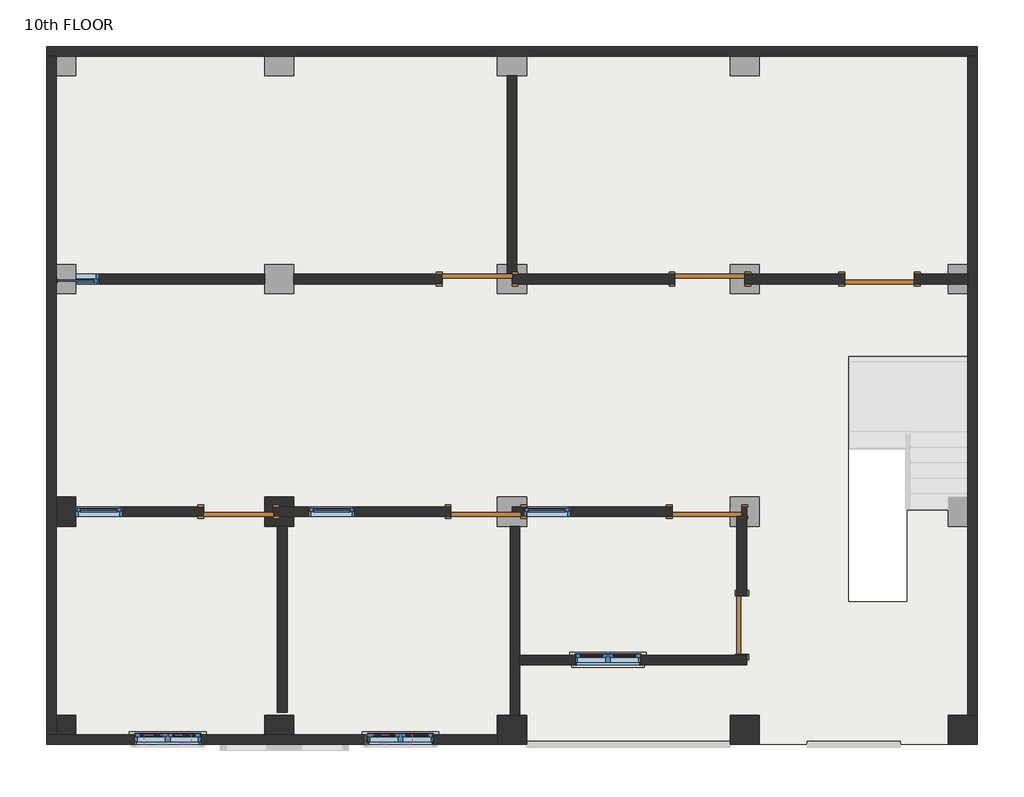
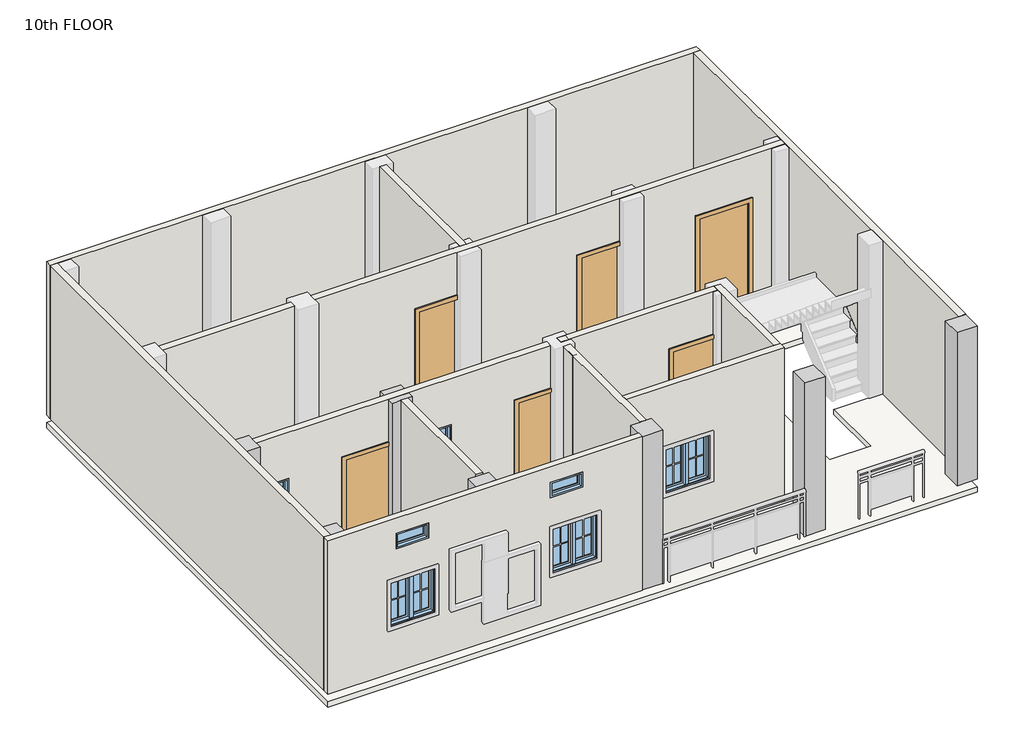
# One storey, part 1 of 2: 15 walls, 9 windows, 7 columns, 7 doors, 1 slab.
"""IFC4 building model written with IfcOpenShell, lengths in millimetres."""

from ifc_helpers import new_model, si_unit, frame, origin, place, context, project, spatial, polyline, outline, extrude, faceted_brep, transform, mapped, element, save
from components import door_e00f436c, door_a1797ceb, window_4c2727af, window_0bf3737e, window_78893e6c, window_0d9958e7

model = new_model("IFC4")

# Units and contexts
model_context = context("Model", 3, world=origin())
ifc_project = project(units=[si_unit("LENGTHUNIT", "METRE", prefix="MILLI")], contexts=[model_context])

# Site, building, storey
site = spatial("IfcSite", under=ifc_project)
building = spatial("IfcBuilding", under=site)
storey = spatial("IfcBuildingStorey", under=building, Name="10th FLOOR", Elevation=30327.6)

# Columns
placement = place(None, origin())
element("IfcColumn", 1, ObjectType="column family : column family", at=placement, inside=storey, context=model_context, shape_type="Brep", body=[
    faceted_brep([(-12576.097125, 2486.2065522, 30332.6), (-12957.097125, 2486.2065522, 30332.6), (-12957.097125, 2867.2065522, 30332.6), (-12576.097125, 2867.2065522, 30332.6), (-12576.097125, 2740.2065522, 30332.6), (-12842.797125, 2740.2065522, 30332.6), (-12842.797125, 2613.2065522, 30332.6), (-12576.097125, 2613.2065522, 30332.6), (-12576.097125, 2486.2065522, 33370.6), (-12576.097125, 2613.2065522, 33370.6), (-12957.097125, 2486.2065522, 33370.6), (-12957.097125, 2613.2065522, 33370.6), (-12957.097125, 2613.2065522, 32461.2), (-12957.097125, 2740.2065522, 32461.2), (-12957.097125, 2740.2065522, 33370.6), (-12957.097125, 2867.2065522, 33370.6), (-12576.097125, 2867.2065522, 33370.6), (-12842.797125, 2613.2065522, 32461.2), (-12842.797125, 2740.2065522, 32461.2), (-12576.097125, 2740.2065522, 33370.6)], [[[0, 1, 2, 3, 4, 5, 6, 7]], [[8, 0, 7, 9]], [[1, 0, 8, 10]], [[2, 1, 10, 11, 12, 13, 14, 15]], [[3, 2, 15, 16]], [[10, 8, 9, 11]], [[6, 17, 12, 11, 9, 7]], [[13, 18, 5, 4, 19, 14]], [[3, 16, 19, 4]], [[16, 15, 14, 19]], [[17, 18, 13, 12]], [[18, 17, 6, 5]]]),
])
element("IfcColumn", 2, ObjectType="column family : column family", at=placement, inside=storey, context=model_context, shape_type="SweptSolid", body=[
    extrude(outline(polyline([(-15433.597125, 2867.2065522), (-15433.597125, 2486.2065522), (-15687.597125, 2486.2065522), (-15687.597125, 2867.2065522), (-15433.597125, 2867.2065522)])), frame((0.0, 0.0, 30332.6), z_axis=(0.0, 0.0, 1.0), x_axis=(1.0, 0.0, 0.0)), (0.0, 0.0, 1.0), 3038.0),
])
element("IfcColumn", 3, ObjectType="column family : column family", at=placement, inside=storey, context=model_context, shape_type="SweptSolid", body=[
    extrude(outline(polyline([(-15433.597125, 9.7065522), (-15433.597125, -244.2934478), (-15687.597125, -244.2934478), (-15687.597125, 9.7065522), (-15433.597125, 9.7065522)])), frame((0.0, 0.0, 30332.6), z_axis=(0.0, 0.0, 1.0), x_axis=(1.0, 0.0, 0.0)), (0.0, 0.0, 1.0), 3038.0),
])
element("IfcColumn", 4, ObjectType="column family : column family", at=placement, inside=storey, context=model_context, shape_type="SweptSolid", body=[
    extrude(outline(polyline([(-3622.597125, 9.7065522), (-3622.597125, -371.2934478), (-4003.597125, -371.2934478), (-4003.597125, 9.7065522), (-3622.597125, 9.7065522)])), frame((0.0, 0.0, 30332.6), z_axis=(0.0, 0.0, 1.0), x_axis=(1.0, 0.0, 0.0)), (0.0, 0.0, 1.0), 3038.0),
])
element("IfcColumn", 5, ObjectType="column family : column family", at=placement, inside=storey, context=model_context, shape_type="SweptSolid", body=[
    extrude(outline(polyline([(-6480.097125, 9.7065522), (-6480.097125, -371.2934478), (-6861.097125, -371.2934478), (-6861.097125, 9.7065522), (-6480.097125, 9.7065522)])), frame((0.0, 0.0, 30332.6), z_axis=(0.0, 0.0, 1.0), x_axis=(1.0, 0.0, 0.0)), (0.0, 0.0, 1.0), 3038.0),
])
element("IfcColumn", 6, ObjectType="column family : column family", at=placement, inside=storey, context=model_context, shape_type="SweptSolid", body=[
    extrude(outline(polyline([(-9528.097125, 9.7065522), (-9528.097125, -371.2934478), (-9909.097125, -371.2934478), (-9909.097125, 9.7065522), (-9528.097125, 9.7065522)])), frame((0.0, 0.0, 30332.6), z_axis=(0.0, 0.0, 1.0), x_axis=(1.0, 0.0, 0.0)), (0.0, 0.0, 1.0), 3038.0),
])
element("IfcColumn", 7, ObjectType="column family : column family", at=placement, inside=storey, context=model_context, shape_type="SweptSolid", body=[
    extrude(outline(polyline([(-12957.097125, 9.7065522), (-12576.097125, 9.7065522), (-12576.097125, -244.2934478), (-12957.097125, -244.2934478), (-12957.097125, 9.7065522)])), frame((0.0, 0.0, 30332.6), z_axis=(0.0, 0.0, 1.0), x_axis=(1.0, 0.0, 0.0)), (0.0, 0.0, 1.0), 3038.0),
])

# Doors
door_shape = door_e00f436c(model_context)
element("IfcDoor", 8, ObjectType="Single-Flush : 30\" x 80\"", at=placement, inside=storey, context=model_context, shape_type="MappedRepresentation", body=[
    mapped(door_shape, transform((-6708.697125, 1190.8065522, 30327.6), x_axis=(0.0, -1.0, 0.0), y_axis=(1.0, 0.0, 0.0), z_axis=(0.0, 0.0, 1.0))),
])
door_2_shape = door_a1797ceb(model_context)
element("IfcDoor", 9, ObjectType="Single-Flush : 36\" x 84\"", at=placement, inside=storey, context=model_context, shape_type="MappedRepresentation", body=[
    mapped(door_2_shape, transform((-10175.797125, 5724.7065522, 30327.6), x_axis=(1.0, 0.0, 0.0), y_axis=(0.0, 1.0, 0.0), z_axis=(0.0, 0.0, 1.0))),
])
element("IfcDoor", 10, ObjectType="Single-Flush : 36\" x 84\"", at=placement, inside=storey, context=model_context, shape_type="MappedRepresentation", body=[
    mapped(door_2_shape, transform((-10061.497125, 2676.7065522, 30327.6), x_axis=(-1.0, 0.0, 0.0), y_axis=(0.0, -1.0, 0.0), z_axis=(0.0, 0.0, 1.0))),
])
element("IfcDoor", 11, ObjectType="Single-Flush : 36\" x 84\"", at=placement, inside=storey, context=model_context, shape_type="MappedRepresentation", body=[
    mapped(door_2_shape, transform((-13299.997125, 2676.7065522, 30327.6), x_axis=(-1.0, 0.0, 0.0), y_axis=(0.0, -1.0, 0.0), z_axis=(0.0, 0.0, 1.0))),
])
element("IfcDoor", 12, ObjectType="Single-Flush : 36\" x 84\"", at=placement, inside=storey, context=model_context, shape_type="MappedRepresentation", body=[
    mapped(door_2_shape, transform((-7127.797125, 5724.7065522, 30327.6), x_axis=(1.0, 0.0, 0.0), y_axis=(0.0, 1.0, 0.0), z_axis=(0.0, 0.0, 1.0))),
])
element("IfcDoor", 13, ObjectType="Single-Flush : 36\" x 84\"", at=placement, inside=storey, context=model_context, shape_type="MappedRepresentation", body=[
    mapped(door_2_shape, transform((-7165.897125, 2676.7065522, 30327.6), x_axis=(-1.0, 0.0, 0.0), y_axis=(0.0, -1.0, 0.0), z_axis=(0.0, 0.0, 1.0))),
])
element("IfcDoor", 14, ObjectType="Single-Flush : 36\" x 84\"", at=placement, inside=storey, context=model_context, shape_type="MappedRepresentation", body=[
    mapped(door_2_shape, transform((-4905.297125, 5724.7065522, 30327.6), x_axis=(-1.0, 0.0, 0.0), y_axis=(0.0, -1.0, 0.0), z_axis=(0.0, 0.0, 1.0))),
])

# Slab
element("IfcSlab", 15, ObjectType="Generic - 4\"", at=placement, inside=storey, context=model_context, shape_type="SweptSolid", body=[
    extrude(outline(polyline([(-3622.597125, 8772.7065522), (-3622.597125, -371.2934478), (-15814.597125, -371.2934478), (-15814.597125, 8772.7065522), (-3622.597125, 8772.7065522)]), holes=[polyline([(-3734.357125, 4711.0719226), (-5310.2646464, 4711.0719226), (-5310.2646464, 1502.3126957), (-4547.7736682, 1502.3126957), (-4547.7736682, 2699.911213), (-3734.357125, 2699.911213), (-3734.357125, 4711.0719226)])]), frame((0.0, 0.0, 30073.6), z_axis=(0.0, 0.0, 1.0), x_axis=(1.0, 0.0, 0.0)), (0.0, 0.0, 1.0), 101.6),
])

# Walls
element("IfcWall", 16, ObjectType="Generic - 5\"", at=placement, inside=storey, context=model_context, shape_type="Brep", body=[
    faceted_brep([(-15814.597125, 8645.7065522, 30327.6), (-15687.597125, 8645.7065522, 30327.6), (-3749.597125, 8645.7065522, 30327.6), (-3622.597125, 8645.7065522, 30327.6), (-3622.597125, 8645.7065522, 33375.6), (-3749.597125, 8645.7065522, 33375.6), (-15687.597125, 8645.7065522, 33375.6), (-15814.597125, 8645.7065522, 33375.6), (-15814.597125, 8772.7065522, 30327.6), (-15814.597125, 8772.7065522, 33375.6), (-3622.597125, 8772.7065522, 33375.6), (-3622.597125, 8772.7065522, 30327.6)], [[[0, 1, 2, 3, 4, 5, 6, 7]], [[8, 9, 10, 11]], [[3, 2, 1, 0, 8, 11]], [[7, 6, 5, 4, 10, 9]], [[4, 3, 11, 10]], [[0, 7, 9, 8]]]),
])
element("IfcWall", 17, ObjectType="Generic - 5\"", at=placement, inside=storey, context=model_context, shape_type="Brep", body=[
    faceted_brep([(-3749.597125, 8645.7065522, 30327.6), (-3749.597125, 5788.2065522, 30327.6), (-3749.597125, 5661.2065522, 30327.6), (-3749.597125, 9.7065522, 30327.6), (-3749.597125, 9.7065522, 33375.6), (-3749.597125, 5661.2065522, 33375.6), (-3749.597125, 5788.2065522, 33375.6), (-3749.597125, 8645.7065522, 33375.6), (-3622.597125, 8645.7065522, 30327.6), (-3622.597125, 8645.7065522, 33375.6), (-3622.597125, 9.7065522, 33375.6), (-3622.597125, 9.7065522, 33370.6), (-3622.597125, 9.7065522, 30332.6), (-3622.597125, 9.7065522, 30327.6)], [[[0, 1, 2, 3, 4, 5, 6, 7]], [[8, 9, 10, 11, 12, 13]], [[3, 2, 1, 0, 8, 13]], [[4, 3, 13, 12, 11, 10]], [[7, 6, 5, 4, 10, 9]], [[0, 7, 9, 8]]]),
])
element("IfcWall", 18, ObjectType="Generic - 5\"", at=placement, inside=storey, context=model_context, shape_type="Brep", body=[
    faceted_brep([(-9909.097125, -244.2934478, 30327.6), (-15687.597125, -244.2934478, 30327.6), (-15814.597125, -244.2934478, 30327.6), (-15814.597125, -244.2934478, 33375.6), (-15687.597125, -244.2934478, 33375.6), (-9909.097125, -244.2934478, 33375.6), (-13795.297125, -244.2934478, 32156.4), (-14658.897125, -244.2934478, 32156.4), (-14658.897125, -244.2934478, 31242.0), (-13795.297125, -244.2934478, 31242.0), (-10747.297125, -244.2934478, 32156.4), (-11610.897125, -244.2934478, 32156.4), (-11610.897125, -244.2934478, 31242.0), (-10747.297125, -244.2934478, 31242.0), (-13922.297125, -244.2934478, 33070.8), (-14531.897125, -244.2934478, 33070.8), (-14531.897125, -244.2934478, 32766.0), (-13922.297125, -244.2934478, 32766.0), (-11026.697125, -244.2934478, 33070.8), (-11636.297125, -244.2934478, 33070.8), (-11636.297125, -244.2934478, 32766.0), (-11026.697125, -244.2934478, 32766.0), (-9909.097125, -371.2934478, 30327.6), (-9909.097125, -371.2934478, 30332.6), (-9909.097125, -371.2934478, 33370.6), (-9909.097125, -371.2934478, 33375.6), (-15814.597125, -371.2934478, 33375.6), (-15814.597125, -371.2934478, 30327.6), (-13795.297125, -371.2934478, 32156.4), (-13795.297125, -371.2934478, 31242.0), (-14658.897125, -371.2934478, 31242.0), (-14658.897125, -371.2934478, 32156.4), (-10747.297125, -371.2934478, 32156.4), (-10747.297125, -371.2934478, 31242.0), (-11610.897125, -371.2934478, 31242.0), (-11610.897125, -371.2934478, 32156.4), (-13922.297125, -371.2934478, 33070.8), (-13922.297125, -371.2934478, 32766.0), (-14531.897125, -371.2934478, 32766.0), (-14531.897125, -371.2934478, 33070.8), (-11026.697125, -371.2934478, 33070.8), (-11026.697125, -371.2934478, 32766.0), (-11636.297125, -371.2934478, 32766.0), (-11636.297125, -371.2934478, 33070.8)], [[[0, 1, 2, 3, 4, 5], [6, 7, 8, 9], [10, 11, 12, 13], [14, 15, 16, 17], [18, 19, 20, 21]], [[22, 23, 24, 25, 26, 27], [28, 29, 30, 31], [32, 33, 34, 35], [36, 37, 38, 39], [40, 41, 42, 43]], [[2, 1, 0, 22, 27]], [[5, 4, 3, 26, 25]], [[0, 5, 25, 24, 23, 22]], [[3, 2, 27, 26]], [[29, 28, 6, 9]], [[30, 29, 9, 8]], [[31, 30, 8, 7]], [[28, 31, 7, 6]], [[33, 32, 10, 13]], [[34, 33, 13, 12]], [[35, 34, 12, 11]], [[32, 35, 11, 10]], [[37, 36, 14, 17]], [[38, 37, 17, 16]], [[39, 38, 16, 15]], [[36, 39, 15, 14]], [[41, 40, 18, 21]], [[42, 41, 21, 20]], [[43, 42, 20, 19]], [[40, 43, 19, 18]]]),
])
element("IfcWall", 19, ObjectType="Generic - 5\"", at=placement, inside=storey, context=model_context, shape_type="Brep", body=[
    faceted_brep([(-15687.597125, -244.2934478, 30327.6), (-15687.597125, 8645.7065522, 30327.6), (-15687.597125, 8645.7065522, 30332.6), (-15687.597125, 8645.7065522, 33370.6), (-15687.597125, 8645.7065522, 33375.6), (-15687.597125, -244.2934478, 33375.6), (-15687.597125, -244.2934478, 33370.6), (-15687.597125, -244.2934478, 30332.6), (-15814.597125, -244.2934478, 30327.6), (-15814.597125, -244.2934478, 33375.6), (-15814.597125, 8645.7065522, 33375.6), (-15814.597125, 8645.7065522, 30327.6)], [[[0, 1, 2, 3, 4, 5, 6, 7]], [[8, 9, 10, 11]], [[1, 0, 8, 11]], [[5, 4, 10, 9]], [[4, 3, 2, 1, 11, 10]], [[0, 7, 6, 5, 9, 8]]]),
])
element("IfcWall", 20, ObjectType="Generic - 5\"", at=placement, inside=storey, context=model_context, shape_type="SweptSolid", body=[
    extrude(outline(polyline([(30327.6, -15433.597125), (30327.6, -12957.097125), (33375.6, -12957.097125), (33375.6, -15433.597125), (32461.2, -15433.597125), (32461.2, -15128.797125), (30632.4, -15128.797125), (30632.4, -15433.597125), (30327.6, -15433.597125)])), frame((0.0, 5661.2065522, 0.0), z_axis=(0.0, 1.0, 0.0), x_axis=(0.0, 0.0, 1.0)), (0.0, 0.0, 1.0), 127.0),
])
element("IfcWall", 21, ObjectType="Generic - 5\"", at=placement, inside=storey, context=model_context, shape_type="Brep", body=[
    faceted_brep([(-9782.097125, 8391.7065522, 30327.6), (-9782.097125, 5788.2065522, 30327.6), (-9782.097125, 5788.2065522, 30332.6), (-9782.097125, 5788.2065522, 32461.2), (-9782.097125, 5788.2065522, 33370.6), (-9782.097125, 5788.2065522, 33375.6), (-9782.097125, 8391.7065522, 33375.6), (-9655.097125, 8391.7065522, 30327.6), (-9655.097125, 8391.7065522, 33375.6), (-9655.097125, 5788.2065522, 33375.6), (-9655.097125, 5788.2065522, 33370.6), (-9655.097125, 5788.2065522, 30332.6), (-9655.097125, 5788.2065522, 30327.6), (-9718.597125, 5788.2065522, 30327.6)], [[[0, 1, 2, 3, 4, 5, 6]], [[7, 8, 9, 10, 11, 12]], [[1, 0, 7, 12, 13]], [[6, 5, 9, 8]], [[0, 6, 8, 7]], [[5, 4, 3, 2, 1, 13, 12, 11, 10, 9]]]),
])
element("IfcWall", 22, ObjectType="Generic - 5\"", at=placement, inside=storey, context=model_context, shape_type="Brep", body=[
    faceted_brep([(-6670.597125, 5661.2065522, 30327.6), (-5362.497125, 5661.2065522, 30327.6), (-5362.497125, 5661.2065522, 32461.2), (-4448.097125, 5661.2065522, 32461.2), (-4448.097125, 5661.2065522, 30327.6), (-3749.597125, 5661.2065522, 30327.6), (-3749.597125, 5661.2065522, 30332.6), (-3749.597125, 5661.2065522, 33370.6), (-3749.597125, 5661.2065522, 33375.6), (-12576.097125, 5661.2065522, 33375.6), (-12576.097125, 5661.2065522, 30327.6), (-10632.997125, 5661.2065522, 30327.6), (-10632.997125, 5661.2065522, 32461.2), (-9909.097125, 5661.2065522, 32461.2), (-9718.597125, 5661.2065522, 32461.2), (-9718.597125, 5661.2065522, 30332.6), (-9718.597125, 5661.2065522, 30327.6), (-7584.997125, 5661.2065522, 30327.6), (-7584.997125, 5661.2065522, 32461.2), (-6861.097125, 5661.2065522, 32461.2), (-6670.597125, 5661.2065522, 32461.2), (-6670.597125, 5661.2065522, 30332.6), (-5362.497125, 5788.2065522, 32461.2), (-5362.497125, 5788.2065522, 30327.6), (-6670.597125, 5788.2065522, 30327.6), (-6670.597125, 5788.2065522, 30332.6), (-6670.597125, 5788.2065522, 32461.2), (-6861.097125, 5788.2065522, 32461.2), (-7584.997125, 5788.2065522, 32461.2), (-7584.997125, 5788.2065522, 30327.6), (-9655.097125, 5788.2065522, 30327.6), (-9718.597125, 5788.2065522, 30327.6), (-9718.597125, 5788.2065522, 30332.6), (-9718.597125, 5788.2065522, 32461.2), (-9782.097125, 5788.2065522, 32461.2), (-9909.097125, 5788.2065522, 32461.2), (-10632.997125, 5788.2065522, 32461.2), (-10632.997125, 5788.2065522, 30327.6), (-12576.097125, 5788.2065522, 30327.6), (-12576.097125, 5788.2065522, 33375.6), (-9782.097125, 5788.2065522, 33375.6), (-9655.097125, 5788.2065522, 33375.6), (-3749.597125, 5788.2065522, 33375.6), (-3749.597125, 5788.2065522, 33370.6), (-3749.597125, 5788.2065522, 30332.6), (-3749.597125, 5788.2065522, 30327.6), (-4448.097125, 5788.2065522, 30327.6), (-4448.097125, 5788.2065522, 32461.2)], [[[0, 1, 2, 3, 4, 5, 6, 7, 8, 9, 10, 11, 12, 13, 14, 15, 16, 17, 18, 19, 20, 21]], [[22, 23, 24, 25, 26, 27, 28, 29, 30, 31, 32, 33, 34, 35, 36, 37, 38, 39, 40, 41, 42, 43, 44, 45, 46, 47]], [[11, 10, 38, 37]], [[17, 16, 31, 30, 29]], [[46, 45, 5, 4]], [[24, 23, 1, 0]], [[9, 8, 42, 41, 40, 39]], [[10, 9, 39, 38]], [[8, 7, 6, 5, 45, 44, 43, 42]], [[33, 32, 31, 16, 15, 14]], [[36, 35, 34, 33, 14, 13, 12]], [[37, 36, 12, 11]], [[26, 25, 24, 0, 21, 20]], [[28, 27, 26, 20, 19, 18]], [[29, 28, 18, 17]], [[2, 1, 23, 22]], [[3, 2, 22, 47]], [[4, 3, 47, 46]]]),
])
element("IfcWall", 23, ObjectType="Generic - 5\"", at=placement, inside=storey, context=model_context, shape_type="Brep", body=[
    faceted_brep([(-14823.997125, 2613.2065522, 30632.4), (-15433.597125, 2613.2065522, 30632.4), (-15433.597125, 2613.2065522, 30327.6), (-13757.197125, 2613.2065522, 30327.6), (-13757.197125, 2613.2065522, 32461.2), (-12957.097125, 2613.2065522, 32461.2), (-12842.797125, 2613.2065522, 32461.2), (-12842.797125, 2613.2065522, 30332.6), (-12842.797125, 2613.2065522, 30327.6), (-10518.697125, 2613.2065522, 30327.6), (-10518.697125, 2613.2065522, 32461.2), (-9909.097125, 2613.2065522, 32461.2), (-9909.097125, 2613.2065522, 33375.6), (-15433.597125, 2613.2065522, 33375.6), (-15433.597125, 2613.2065522, 32461.2), (-14823.997125, 2613.2065522, 32461.2), (-12385.597125, 2613.2065522, 32461.2), (-11775.997125, 2613.2065522, 32461.2), (-11775.997125, 2613.2065522, 30632.4), (-12385.597125, 2613.2065522, 30632.4), (-15433.597125, 2740.2065522, 30327.6), (-15433.597125, 2740.2065522, 30632.4), (-14823.997125, 2740.2065522, 30632.4), (-14823.997125, 2740.2065522, 32461.2), (-15433.597125, 2740.2065522, 32461.2), (-15433.597125, 2740.2065522, 33375.6), (-9909.097125, 2740.2065522, 33375.6), (-9909.097125, 2740.2065522, 32461.2), (-10518.697125, 2740.2065522, 32461.2), (-10518.697125, 2740.2065522, 30327.6), (-12842.797125, 2740.2065522, 30327.6), (-12842.797125, 2740.2065522, 30332.6), (-12842.797125, 2740.2065522, 32461.2), (-12957.097125, 2740.2065522, 32461.2), (-13757.197125, 2740.2065522, 32461.2), (-13757.197125, 2740.2065522, 30327.6), (-12385.597125, 2740.2065522, 32461.2), (-12385.597125, 2740.2065522, 30632.4), (-11775.997125, 2740.2065522, 30632.4), (-11775.997125, 2740.2065522, 32461.2)], [[[0, 1, 2, 3, 4, 5, 6, 7, 8, 9, 10, 11, 12, 13, 14, 15], [16, 17, 18, 19]], [[20, 21, 22, 23, 24, 25, 26, 27, 28, 29, 30, 31, 32, 33, 34, 35], [36, 37, 38, 39]], [[30, 29, 9, 8]], [[20, 35, 3, 2]], [[26, 12, 11, 27]], [[13, 12, 26, 25]], [[14, 13, 25, 24]], [[2, 1, 21, 20]], [[28, 10, 9, 29]], [[10, 28, 27, 11]], [[4, 3, 35, 34]], [[6, 5, 4, 34, 33, 32]], [[8, 7, 6, 32, 31, 30]], [[22, 21, 1, 0]], [[23, 22, 0, 15]], [[24, 23, 15, 14]], [[37, 36, 16, 19]], [[38, 37, 19, 18]], [[39, 38, 18, 17]], [[36, 39, 17, 16]]]),
])
element("IfcWall", 24, ObjectType="Generic - 5\"", at=placement, inside=storey, context=model_context, shape_type="Brep", body=[
    faceted_brep([(-9616.997125, 9.7065522, 30327.6), (-9616.997125, 670.1065522, 30327.6), (-9616.997125, 797.1065522, 30327.6), (-9616.997125, 2486.2065522, 30327.6), (-9616.997125, 2486.2065522, 33375.6), (-9616.997125, 797.1065522, 33375.6), (-9616.997125, 670.1065522, 33375.6), (-9616.997125, 9.7065522, 33375.6), (-9743.997125, 9.7065522, 30327.6), (-9743.997125, 9.7065522, 33375.6), (-9743.997125, 2486.2065522, 33375.6), (-9743.997125, 2486.2065522, 30327.6)], [[[0, 1, 2, 3, 4, 5, 6, 7]], [[8, 9, 10, 11]], [[3, 2, 1, 0, 8, 11]], [[4, 3, 11, 10]], [[7, 6, 5, 4, 10, 9]], [[0, 7, 9, 8]]]),
])
element("IfcWall", 25, ObjectType="Generic - 5\"", at=placement, inside=storey, context=model_context, shape_type="SweptSolid", body=[
    extrude(outline(polyline([(-9743.997125, 2181.4065522), (-9743.997125, 2486.2065522), (-9616.997125, 2486.2065522), (-9616.997125, 2181.4065522), (-9743.997125, 2181.4065522)])), frame((0.0, 0.0, 30327.6), z_axis=(0.0, 0.0, 1.0), x_axis=(1.0, 0.0, 0.0)), (0.0, 0.0, 1.0), 3048.0),
])
element("IfcWall", 26, ObjectType="Generic - 5\"", at=placement, inside=storey, context=model_context, shape_type="Brep", body=[
    faceted_brep([(-6772.197125, 2613.2065522, 33375.6), (-9718.597125, 2613.2065522, 33375.6), (-9718.597125, 2613.2065522, 33370.6), (-9718.597125, 2613.2065522, 30332.6), (-9718.597125, 2613.2065522, 30327.6), (-7623.097125, 2613.2065522, 30327.6), (-7623.097125, 2613.2065522, 32461.2), (-6861.097125, 2613.2065522, 32461.2), (-6772.197125, 2613.2065522, 32461.2), (-6772.197125, 2613.2065522, 33370.6), (-9566.197125, 2613.2065522, 32461.2), (-9528.097125, 2613.2065522, 32461.2), (-8956.597125, 2613.2065522, 32461.2), (-8956.597125, 2613.2065522, 30632.4), (-9528.097125, 2613.2065522, 30632.4), (-9566.197125, 2613.2065522, 30632.4), (-9718.597125, 2740.2065522, 33375.6), (-6772.197125, 2740.2065522, 33375.6), (-6772.197125, 2740.2065522, 32461.2), (-6861.097125, 2740.2065522, 32461.2), (-7623.097125, 2740.2065522, 32461.2), (-7623.097125, 2740.2065522, 30327.6), (-9718.597125, 2740.2065522, 30327.6), (-9718.597125, 2740.2065522, 30332.6), (-9718.597125, 2740.2065522, 33370.6), (-9566.197125, 2740.2065522, 32461.2), (-9566.197125, 2740.2065522, 30632.4), (-9528.097125, 2740.2065522, 30632.4), (-8956.597125, 2740.2065522, 30632.4), (-8956.597125, 2740.2065522, 32461.2), (-9528.097125, 2740.2065522, 32461.2)], [[[0, 1, 2, 3, 4, 5, 6, 7, 8, 9], [10, 11, 12, 13, 14, 15]], [[16, 17, 18, 19, 20, 21, 22, 23, 24], [25, 26, 27, 28, 29, 30]], [[4, 22, 21, 5]], [[1, 0, 17, 16]], [[4, 3, 2, 1, 16, 24, 23, 22]], [[26, 25, 10, 15]], [[28, 27, 26, 15, 14, 13]], [[29, 28, 13, 12]], [[25, 30, 29, 12, 11, 10]], [[20, 6, 5, 21]], [[6, 20, 19, 18, 8, 7]], [[17, 0, 9, 8, 18]]]),
])
element("IfcWall", 27, ObjectType="Generic - 5\"", at=placement, inside=storey, context=model_context, shape_type="Brep", body=[
    faceted_brep([(-6645.197125, 797.1065522, 30327.6), (-6645.197125, 809.8065522, 30327.6), (-6645.197125, 809.8065522, 32359.6), (-6645.197125, 1571.8065522, 32359.6), (-6645.197125, 1571.8065522, 30327.6), (-6645.197125, 2740.2065522, 30327.6), (-6645.197125, 2740.2065522, 30332.6), (-6645.197125, 2740.2065522, 33370.6), (-6645.197125, 2740.2065522, 33375.6), (-6645.197125, 797.1065522, 33375.6), (-6772.197125, 809.8065522, 32359.6), (-6772.197125, 809.8065522, 30327.6), (-6772.197125, 797.1065522, 30327.6), (-6772.197125, 797.1065522, 33375.6), (-6772.197125, 2613.2065522, 33375.6), (-6772.197125, 2740.2065522, 33375.6), (-6772.197125, 2740.2065522, 32461.2), (-6772.197125, 2613.2065522, 32461.2), (-6772.197125, 2613.2065522, 30332.6), (-6772.197125, 2613.2065522, 30327.6), (-6772.197125, 1571.8065522, 30327.6), (-6772.197125, 1571.8065522, 32359.6), (-6708.697125, 2613.2065522, 30327.6), (-6708.697125, 2740.2065522, 30327.6), (-6708.697125, 2613.2065522, 32461.2), (-6708.697125, 2613.2065522, 30332.6), (-6708.697125, 2740.2065522, 32461.2), (-6708.697125, 2740.2065522, 30332.6)], [[[0, 1, 2, 3, 4, 5, 6, 7, 8, 9]], [[10, 11, 12, 13, 14, 15, 16, 17, 18, 19, 20, 21]], [[20, 19, 22, 23, 5, 4]], [[12, 11, 1, 0]], [[9, 8, 15, 14, 13]], [[24, 25, 22, 19, 18, 17]], [[26, 24, 17, 16]], [[22, 25, 24, 26, 27, 23]], [[8, 7, 6, 5, 23, 27, 26, 16, 15]], [[0, 9, 13, 12]], [[2, 1, 11, 10]], [[3, 2, 10, 21]], [[4, 3, 21, 20]]]),
])
element("IfcWall", 28, ObjectType="Generic - 5\"", at=placement, inside=storey, context=model_context, shape_type="Brep", body=[
    faceted_brep([(-9718.597125, 2613.2065522, 30327.6), (-9566.197125, 2613.2065522, 30327.6), (-9566.197125, 2613.2065522, 30632.4), (-9566.197125, 2613.2065522, 32461.2), (-9566.197125, 2613.2065522, 33375.6), (-9718.597125, 2613.2065522, 33375.6), (-9718.597125, 2613.2065522, 33370.6), (-9718.597125, 2613.2065522, 30332.6), (-9718.597125, 2740.2065522, 30327.6), (-9718.597125, 2740.2065522, 30332.6), (-9718.597125, 2740.2065522, 33370.6), (-9718.597125, 2740.2065522, 33375.6), (-9566.197125, 2740.2065522, 33375.6), (-9566.197125, 2740.2065522, 32461.2), (-9566.197125, 2740.2065522, 30632.4), (-9566.197125, 2740.2065522, 30327.6)], [[[0, 1, 2, 3, 4, 5, 6, 7]], [[8, 9, 10, 11, 12, 13, 14, 15]], [[1, 0, 8, 15]], [[4, 3, 2, 1, 15, 14, 13, 12]], [[5, 4, 12, 11]], [[0, 7, 6, 5, 11, 10, 9, 8]]]),
])
element("IfcWall", 29, ObjectType="Generic - 5\"", at=placement, inside=storey, context=model_context, shape_type="SweptSolid", body=[
    extrude(outline(polyline([(-12791.997125, 47.8065522), (-12791.997125, 2486.2065522), (-12664.997125, 2486.2065522), (-12664.997125, 47.8065522), (-12791.997125, 47.8065522)])), frame((0.0, 0.0, 30327.6), z_axis=(0.0, 0.0, 1.0), x_axis=(1.0, 0.0, 0.0)), (0.0, 0.0, 1.0), 3048.0),
])
element("IfcWall", 30, ObjectType="Generic - 5\"", at=placement, inside=storey, context=model_context, shape_type="Brep", body=[
    faceted_brep([(-9616.997125, 670.1065522, 30327.6), (-6645.197125, 670.1065522, 30327.6), (-6645.197125, 670.1065522, 33375.6), (-9616.997125, 670.1065522, 33375.6), (-8029.497125, 670.1065522, 32156.4), (-8029.497125, 670.1065522, 31242.0), (-8893.097125, 670.1065522, 31242.0), (-8893.097125, 670.1065522, 32156.4), (-9616.997125, 797.1065522, 30327.6), (-9616.997125, 797.1065522, 33375.6), (-6772.197125, 797.1065522, 33375.6), (-6645.197125, 797.1065522, 33375.6), (-6645.197125, 797.1065522, 30327.6), (-6772.197125, 797.1065522, 30327.6), (-8029.497125, 797.1065522, 32156.4), (-8893.097125, 797.1065522, 32156.4), (-8893.097125, 797.1065522, 31242.0), (-8029.497125, 797.1065522, 31242.0)], [[[0, 1, 2, 3], [4, 5, 6, 7]], [[8, 9, 10, 11, 12, 13], [14, 15, 16, 17]], [[1, 0, 8, 13, 12]], [[3, 2, 11, 10, 9]], [[0, 3, 9, 8]], [[2, 1, 12, 11]], [[5, 4, 14, 17]], [[6, 5, 17, 16]], [[7, 6, 16, 15]], [[4, 7, 15, 14]]]),
])

# Windows
window_shape = window_4c2727af(model_context)
element("IfcWindow", 31, ObjectType="Fixed : 24\" x 12\"", at=placement, inside=storey, context=model_context, shape_type="MappedRepresentation", body=[
    mapped(window_shape, transform((-14188.997125, -307.7934478, 31851.6), x_axis=(1.0, 0.0, 0.0), y_axis=(0.0, 1.0, 0.0), z_axis=(0.0, 0.0, 1.0))),
])
element("IfcWindow", 32, ObjectType="Fixed : 24\" x 12\"", at=placement, inside=storey, context=model_context, shape_type="MappedRepresentation", body=[
    mapped(window_shape, transform((-11293.397125, -307.7934478, 31851.6), x_axis=(1.0, 0.0, 0.0), y_axis=(0.0, 1.0, 0.0), z_axis=(0.0, 0.0, 1.0))),
])
window_2_shape = window_0bf3737e(model_context)
element("IfcWindow", 33, ObjectType="Fixed : 24\" x 72\"", at=placement, inside=storey, context=model_context, shape_type="MappedRepresentation", body=[
    mapped(window_2_shape, transform((-15471.697125, 5724.7065522, 30327.6), x_axis=(-1.0, 0.0, 0.0), y_axis=(0.0, -1.0, 0.0), z_axis=(0.0, 0.0, 1.0))),
])
window_3_shape = window_78893e6c(model_context)
element("IfcWindow", 34, ObjectType="Fixed : 24\" x 72\"", at=placement, inside=storey, context=model_context, shape_type="MappedRepresentation", body=[
    mapped(window_3_shape, transform((-15166.897125, 2676.7065522, 30327.6), x_axis=(-1.0, 0.0, 0.0), y_axis=(0.0, -1.0, 0.0), z_axis=(0.0, 0.0, 1.0))),
])
element("IfcWindow", 35, ObjectType="Fixed : 24\" x 72\"", at=placement, inside=storey, context=model_context, shape_type="MappedRepresentation", body=[
    mapped(window_3_shape, transform((-12118.897125, 2676.7065522, 30327.6), x_axis=(-1.0, 0.0, 0.0), y_axis=(0.0, -1.0, 0.0), z_axis=(0.0, 0.0, 1.0))),
])
element("IfcWindow", 36, ObjectType="Fixed : 24\" x 72\"", at=placement, inside=storey, context=model_context, shape_type="MappedRepresentation", body=[
    mapped(window_3_shape, transform((-9299.497125, 2676.7065522, 30327.6), x_axis=(-1.0, 0.0, 0.0), y_axis=(0.0, -1.0, 0.0), z_axis=(0.0, 0.0, 1.0))),
])
window_4_shape = window_0d9958e7(model_context)
element("IfcWindow", 37, ObjectType="Window-Casement-Double : 34\" x 36\"", at=placement, inside=storey, context=model_context, shape_type="MappedRepresentation", body=[
    mapped(window_4_shape, transform((-14227.097125, -307.7934478, 30327.6), x_axis=(1.0, 0.0, 0.0), y_axis=(0.0, 1.0, 0.0), z_axis=(0.0, 0.0, 1.0))),
])
element("IfcWindow", 38, ObjectType="Window-Casement-Double : 34\" x 36\"", at=placement, inside=storey, context=model_context, shape_type="MappedRepresentation", body=[
    mapped(window_4_shape, transform((-11179.097125, -307.7934478, 30327.6), x_axis=(1.0, 0.0, 0.0), y_axis=(0.0, 1.0, 0.0), z_axis=(0.0, 0.0, 1.0))),
])
element("IfcWindow", 39, ObjectType="Window-Casement-Double : 34\" x 36\"", at=placement, inside=storey, context=model_context, shape_type="MappedRepresentation", body=[
    mapped(window_4_shape, transform((-8461.297125, 733.6065522, 30327.6), x_axis=(1.0, 0.0, 0.0), y_axis=(0.0, 1.0, 0.0), z_axis=(0.0, 0.0, 1.0))),
])

save(model, "model.ifc")

# Revit data of these elements
# Type "column family : column family"
#   w2 [instance default] = 0' - 9.88189"
#   w1 [instance default] = 0' - 9.01575"
#   Depth = 1' - 11.62205"
#   Width = 1' - 11.62205"
# Type "Single-Flush : 30\" x 80\""
#   Type Mark = "5"
#   Construction Type Id = "MDOOR"
#   Assembly Code = "C1020"
#   Analytic Construction = "Metal"
#   Thickness = 0' - 2"
#   Heat Transfer Coefficient (U) = 0.651978 BTU/(h·ft²·°F)
#   Height = 6' - 8"
#   Trim Projection Ext = 0' - 1"
#   Trim Projection Int = 0' - 1"
#   Trim Width = 0' - 3"
#   Width = 2' - 6"
#   Define Thermal Properties by = 1
#   Define Thermal Properties by = 1
#   Door Material = Door - Panel
#   Frame Material = Door - Frame
#   Visual Light Transmittance = 0
#   Solar Heat Gain Coefficient = 0
#   Function = (empty or 0)
#   Wall Closure = (empty or 0)
# Type "Single-Flush : 36\" x 84\""
#   Type Mark = "1"
#   Construction Type Id = "MDOOR"
#   Assembly Code = "C1020"
#   Analytic Construction = "Metal"
#   Thickness = 0' - 2"
#   Heat Transfer Coefficient (U) = 0.651978 BTU/(h·ft²·°F)
#   Height = 7' - 0"
#   Trim Projection Ext = 0' - 1"
#   Trim Projection Int = 0' - 1"
#   Trim Width = 0' - 3"
#   Width = 3' - 0"
#   Define Thermal Properties by = 1
#   Define Thermal Properties by = 1
#   Door Material = Door - Panel
#   Frame Material = Door - Frame
#   Visual Light Transmittance = 0
#   Solar Heat Gain Coefficient = 0
#   Function = (empty or 0)
#   Wall Closure = (empty or 0)
# Type "Generic - 4\""
#   Assembly Code = "B1010"
#   Function = 0
#   Layers, outside or top first: 0' - 4" no material (function 1)
# Type "Generic - 5\""
#   Assembly Code = "B2010"
#   Layers, outside or top first: 0' - 5" no material (function 1)
# Type "Fixed : 24\" x 12\""
#   Type Mark = "4"
#   Construction Type Id = "GSP4R"
#   Assembly Code = "B2020100"
#   Analytic Construction = "1/8 in Pilkington single glazing"
#   Visual Light Transmittance = 0.9
#   Solar Heat Gain Coefficient = 0.78
#   Heat Transfer Coefficient (U) = 0.6496 BTU/(h·ft²·°F)
#   Height = 1' - 0"
#   Default Sill Height = 3' - 0"
#   Width = 2' - 0"
#   Window Inset = 0' - 0 3/4"
#   Define Thermal Properties by = 1
#   Define Thermal Properties by = 1
#   Glass Pane Material = Glass
#   Sash Material = Sash
#   Wall Closure = (empty or 0)
# Type "Fixed : 24\" x 72\""
#   Type Mark = "7"
#   Construction Type Id = "GSP4R"
#   Assembly Code = "B2020100"
#   Analytic Construction = "1/8 in Pilkington single glazing"
#   Visual Light Transmittance = 0.9
#   Solar Heat Gain Coefficient = 0.78
#   Heat Transfer Coefficient (U) = 0.6496 BTU/(h·ft²·°F)
#   Height = 6' - 0"
#   Default Sill Height = 1' - 0"
#   Width = 2' - 0"
#   Window Inset = 0' - 0 3/4"
#   Define Thermal Properties by = 1
#   Define Thermal Properties by = 1
#   Glass Pane Material = Glass
#   Sash Material = Sash
#   Wall Closure = (empty or 0)
# Type "Window-Casement-Double : 34\" x 36\""
#   Type Mark = "14"
#   Fire Rating = "0.5h"
#   Assembly Code = "B2020100"
#   Analytic Construction = "Double glazing - domestic"
#   Frame Extension [instance default] = 0' - 0 1/4"
#   Window Inset [instance default] = 0' - 0"
#   Wall Thickness [instance default] = 0' - 6"
#   Interior Wall Closure [instance default] = 0' - 2 1/4"
#   Half Width = 1' - 5"
#   Visual Light Transmittance = 0.81
#   Thermal Resistance (R) = 1.8146 (h·ft²·°F)/BTU
#   Solar Heat Gain Coefficient = 0.76
#   Rough Width = 2' - 10 1/2"
#   Rough Height = 3' - 0 1/2"
#   Height = 3' - 0"
#   Heat Transfer Coefficient (U) = 0.5511 BTU/(h·ft²·°F)
#   Exterior Wall Closure [instance default] = 0' - 1 1/4"
#   Extension Jamb [instance default] = 0' - 2 1/4"
#   Default Sill Height = 3' - 0"
#   Width = 2' - 10"
#   Define Thermal Properties by = 0
#   Muntin Visibility = yes
#   Interior Trim Visibility [instance default] = yes
#   Exterior Trim Visibility [instance default] = yes
#   Extension Jamb Visibility [instance default] = yes
#   Interior Trim Material = Wood - Stained
#   Muntin Pattern = Muntin Pattern_2x2 : Muntin Pattern_2x2
#   Interior Trim = Trim-Window-Interior-Flat : Picture Frame
#   Interior Frame Material = Wood - Stained
#   Glass Panel Material = Glass
#   Exterior Trim Material = Clad - White
#   Exterior Trim = Trim-Window-Exterior-Flat : with Sill
#   Exterior Frame Material = Clad - White
#   Wall Closure = (empty or 0)
# Element 1 (IfcColumn, "column family : column family")
#   w2 = 1' - 3"
#   w1 = 1' - 3"
#   Phase Created = New Construction
#   Materials on its faces: "Default Wall", "inside wall"
# Element 2 (IfcColumn, "column family : column family")
#   w2 = 1' - 3"
#   w1 = 0' - 10"
#   Phase Created = New Construction
#   Materials on its faces: "inside wall", "Default Wall"
# Elements 3, 7 (IfcColumn, "column family : column family")
#   w2 = 1' - 3"
#   w1 = 1' - 3"
#   Phase Created = New Construction
#   Materials on its faces: "Default Wall"
# Element 4 (IfcColumn, "column family : column family")
#   w2 = 1' - 3"
#   w1 = 1' - 3"
#   Phase Created = New Construction
#   Materials on its faces: "Clad - White", "Default Wall"
# Element 5 (IfcColumn, "column family : column family")
#   w2 = 1' - 3"
#   w1 = 1' - 3"
#   Phase Created = New Construction
#   Materials on its faces: "out side wall"
# Element 6 (IfcColumn, "column family : column family")
#   w2 = 1' - 3"
#   w1 = 1' - 3"
#   Phase Created = New Construction
#   Materials on its faces: "out side wall", "Default Wall"
# Element 8 (IfcDoor, "Single-Flush : 30\" x 80\"")
#   Phase Created = New Construction
#   Materials on its faces: "Door - Frame", "Door - Panel"
# Elements 9, 10, 11, 12, 13, 14 (IfcDoor, "Single-Flush : 36\" x 84\"")
#   Phase Created = New Construction
#   Materials on its faces: "Door - Frame", "Door - Panel"
# Element 15 (IfcSlab, "Generic - 4\"")
#   Height Offset From Level = -0' - 6"
#   Phase Created = New Construction
#   Materials on its faces: "Default Floor", "Clad - White", "floor"
# Element 16 (IfcWall, "Generic - 5\"")
#   Top Offset = 0' - 0"
#   Base Offset = 0' - 0"
#   wall height = 10' - 0"
#   Phase Created = New Construction
#   Base Constraint = 10th FLOOR
#   Top Constraint = 11th FLOOR
#   Materials on its faces: "Default Wall", "Clad - White"
# Element 17 (IfcWall, "Generic - 5\"")
#   Top Offset = 0' - 0"
#   Base Offset = 0' - 0"
#   wall height = 10' - 0"
#   Phase Created = New Construction
#   Base Constraint = 10th FLOOR
#   Top Constraint = 11th FLOOR
#   Materials on its faces: "Default Wall", "grey", "Clad - White"
# Element 18 (IfcWall, "Generic - 5\"")
#   Top Offset = 0' - 0"
#   Base Offset = 0' - 0"
#   wall height = 10' - 0"
#   Phase Created = New Construction
#   Base Constraint = 10th FLOOR
#   Top Constraint = 11th FLOOR
#   Materials on its faces: "Default Wall", "out side wall", "Clad - White"
# Element 19 (IfcWall, "Generic - 5\"")
#   Top Offset = 0' - 0"
#   Base Offset = 0' - 0"
#   wall height = 10' - 0"
#   Phase Created = New Construction
#   Base Constraint = 10th FLOOR
#   Top Constraint = 11th FLOOR
#   Materials on its faces: "Default Wall", "inside wall", "Clad - White"
# Elements 20, 23, 26, 27 (IfcWall, "Generic - 5\"")
#   Top Offset = 0' - 0"
#   Base Offset = 0' - 0"
#   wall height = 10' - 0"
#   Phase Created = New Construction
#   Base Constraint = 10th FLOOR
#   Top Constraint = 11th FLOOR
#   Materials on its faces: "Default Wall", "inside wall"
# Elements 21, 25, 28, 29 (IfcWall, "Generic - 5\"")
#   Top Offset = 0' - 0"
#   Base Offset = 0' - 0"
#   wall height = 10' - 0"
#   Phase Created = New Construction
#   Base Constraint = 10th FLOOR
#   Top Constraint = 11th FLOOR
#   Materials on its faces: "Default Wall"
# Elements 22, 24 (IfcWall, "Generic - 5\"")
#   Top Offset = 0' - 0"
#   Base Offset = 0' - 0"
#   wall height = 10' - 0"
#   Phase Created = New Construction
#   Base Constraint = 10th FLOOR
#   Top Constraint = 11th FLOOR
#   Materials on its faces: "Default Wall", "grey"
# Element 30 (IfcWall, "Generic - 5\"")
#   Top Offset = 0' - 0"
#   Base Offset = 0' - 0"
#   wall height = 10' - 0"
#   Phase Created = New Construction
#   Base Constraint = 10th FLOOR
#   Top Constraint = 11th FLOOR
#   Materials on its faces: "Default Wall", "grey", "inside wall"
# Element 31 (IfcWindow, "Fixed : 24\" x 12\"")
#   Mark = "97"
#   Phase Created = New Construction
#   Materials on its faces: "Sash", "Glass"
# Element 32 (IfcWindow, "Fixed : 24\" x 12\"")
#   Mark = "98"
#   Phase Created = New Construction
#   Materials on its faces: "Sash", "Glass"
# Element 33 (IfcWindow, "Fixed : 24\" x 72\"")
#   Mark = "91"
#   Phase Created = New Construction
#   Materials on its faces: "Sash", "Glass"
# Element 34 (IfcWindow, "Fixed : 24\" x 72\"")
#   Mark = "92"
#   Phase Created = New Construction
#   Materials on its faces: "Sash", "Glass"
# Element 35 (IfcWindow, "Fixed : 24\" x 72\"")
#   Mark = "93"
#   Phase Created = New Construction
#   Materials on its faces: "Sash", "Glass"
# Element 36 (IfcWindow, "Fixed : 24\" x 72\"")
#   Mark = "94"
#   Phase Created = New Construction
#   Materials on its faces: "Sash", "Glass"
# Element 37 (IfcWindow, "Window-Casement-Double : 34\" x 36\"")
#   Mark = "95"
#   Window Inset = 0' - 0"
#   Interior Wall Closure = 0' - 2 1/4"
#   Frame Extension = 0' - 0 1/4"
#   Exterior Wall Closure = 0' - 1 1/4"
#   Interior Trim Visibility = yes
#   Exterior Trim Visibility = yes
#   Phase Created = New Construction
#   Materials on its faces: "Wood - Stained", "Glass", "Clad - White"
# Element 38 (IfcWindow, "Window-Casement-Double : 34\" x 36\"")
#   Mark = "96"
#   Window Inset = 0' - 0"
#   Interior Wall Closure = 0' - 2 1/4"
#   Frame Extension = 0' - 0 1/4"
#   Exterior Wall Closure = 0' - 1 1/4"
#   Interior Trim Visibility = yes
#   Exterior Trim Visibility = yes
#   Phase Created = New Construction
#   Materials on its faces: "Wood - Stained", "Glass", "Clad - White"
# Element 39 (IfcWindow, "Window-Casement-Double : 34\" x 36\"")
#   Mark = "99"
#   Window Inset = 0' - 0"
#   Interior Wall Closure = 0' - 2 1/4"
#   Frame Extension = 0' - 0 1/4"
#   Exterior Wall Closure = 0' - 1 1/4"
#   Interior Trim Visibility = yes
#   Exterior Trim Visibility = yes
#   Phase Created = New Construction
#   Materials on its faces: "Wood - Stained", "Glass", "Clad - White"
# Materials
#   "Door - Panel": class "Wood", colour RGB 210 159 95, transparency 0, Cost = 0
#   "Door - Frame": colour RGB 118 70 51, transparency 0, Cost = 0
#   "Glass": class "Glass", colour RGB 0 128 192, transparency 0.75, Description = "Soda Lime Glass", Cost = 0
#   "Sash": class "Wood", colour RGB 224 178 126, transparency 0, Cost = 0
#   "Wood - Stained": class "Wood", colour RGB 224 178 126, transparency 0, Cost = 0
#   "Clad - White": class "Wood", colour RGB 242 242 238, transparency 0, Cost = 0
#   "Default Wall": colour RGB 128 128 128, transparency 0, Cost = 0
#   "inside wall": class "Generic", colour RGB 199 224 95, transparency 0, Cost = 0
#   "out side wall": class "Generic", colour RGB 16 106 159, transparency 0, Cost = 0
#   "Default Floor": colour RGB 128 128 128, transparency 0, Cost = 0
#   "floor": class "Generic", colour RGB 255 255 255, transparency 0, Cost = 0
#   "grey": class "Generic", colour RGB 80 80 80, transparency 0, Cost = 0
